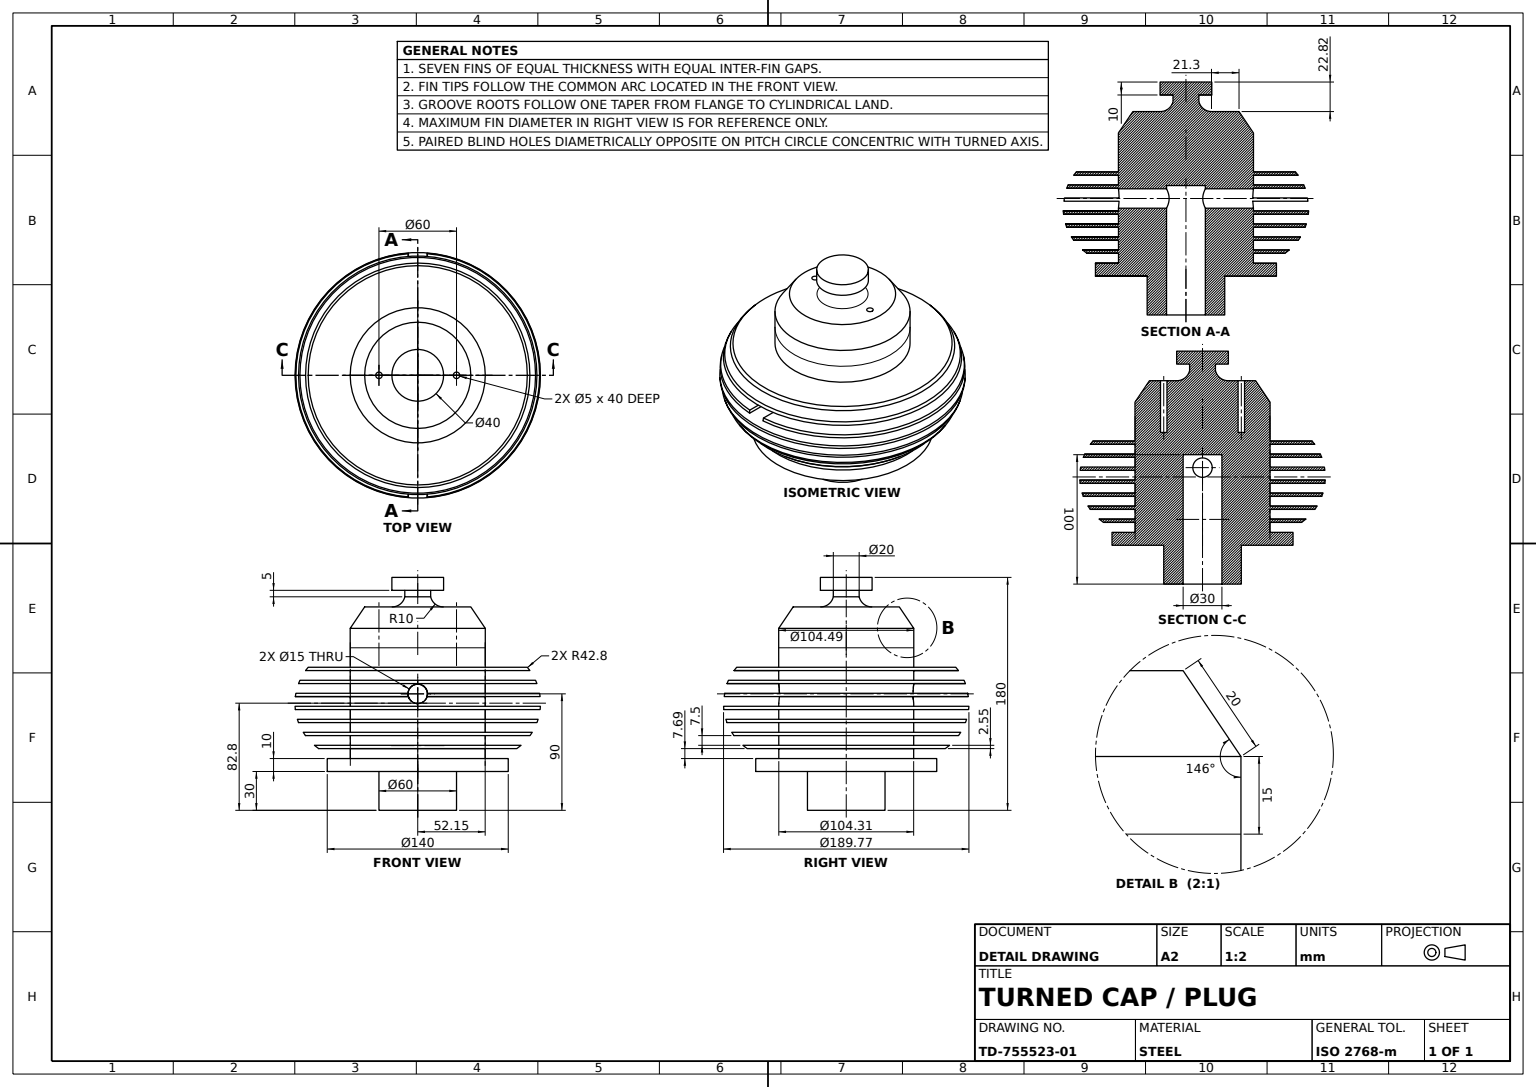
from build123d import *

# Parameters (mm, degrees)
CUT_30_SKETCH_R               = 15
CUT_30_DEPTH                  = 100
RECTANGULAR_CUT_SKETCH_R      = 2.5
RECTANGULAR_CUT_40_DEEP_DEPTH = 40
FRONT_PLANE_CUT_DEPTH         = 204.841147396
FRONT_PLANE_CUT_DEPTH_BACK    = 204.841147396
FRONT_PLANE_CUT_SKETCH_R      = 7.5


with BuildPart() as part:
    # Turned Body Profile → Turned Body (revolve)
    with BuildSketch(Plane.XY, mode=Mode.PRIVATE) as turned_body_sk:
        with BuildLine():
            Line((20, 26.558355194), (0, 26.558355194))
            Line((0, 26.558355194), (0, -153.441644806))
            Line((0, -153.441644806), (30, -153.441644806))
            Line((30, -153.441644806), (30, -123.441644806))
            Line((30, -123.441644806), (70, -123.441644806))
            Line((70, -123.441644806), (70, -113.441644806))
            Line((70, -113.441644806), (52.154011426, -113.441644806))
            Line((52.154011426, -113.441644806), (52.162025925, -105.749506337))
            Line((52.162025925, -105.749506337), (76.634167854, -105.749506337))
            ThreePointArc((76.634167854, -105.749506337), (78.316646551, -104.51429636), (79.93690532, -103.198530512))
            Line((79.93690532, -103.198530512), (52.164683807, -103.198530512))
            Line((52.164683807, -103.198530512), (52.17249811, -95.698535939))
            Line((52.17249811, -95.698535939), (86.852602272, -95.698535939))
            ThreePointArc((86.852602272, -95.698535939), (87.728678054, -94.438348239), (88.559008008, -93.147560114))
            Line((88.559008008, -93.147560114), (52.175155992, -93.147560114))
            Line((52.175155992, -93.147560114), (52.182970295, -85.647565542))
            Line((52.182970295, -85.647565542), (92.237204199, -85.647565542))
            ThreePointArc((92.237204199, -85.647565542), (92.689531284, -84.378879966), (93.101714014, -83.096589717))
            Line((93.101714014, -83.096589717), (52.185628177, -83.096589717))
            Line((52.185628177, -83.096589717), (52.19344248, -75.596595145))
            Line((52.19344248, -75.596595145), (94.666226931, -75.596595145))
            ThreePointArc((94.666226931, -75.596595145), (94.795416565, -74.322754392), (94.88644532, -73.04561932))
            Line((94.88644532, -73.04561932), (52.196100362, -73.04561932))
            Line((52.196100362, -73.04561932), (52.203914665, -65.545624748))
            Line((52.203914665, -65.545624748), (94.649547422, -65.545624748))
            ThreePointArc((94.649547422, -65.545624748), (94.476664711, -64.267241391), (94.265333585, -62.994648923))
            Line((94.265333585, -62.994648923), (52.206572547, -62.994648923))
            Line((52.206572547, -62.994648923), (52.21438685, -55.49465435))
            Line((52.21438685, -55.49465435), (92.184108605, -55.49465435))
            ThreePointArc((92.184108605, -55.49465435), (91.674398419, -54.210606739), (91.123512187, -52.943678525))
            Line((91.123512187, -52.943678525), (52.217044732, -52.943678525))
            Line((52.217044732, -52.943678525), (52.224859035, -45.443683953))
            Line((52.224859035, -45.443683953), (86.750294013, -45.443683953))
            ThreePointArc((86.750294013, -45.443683953), (85.769276316, -44.149118192), (84.73984444, -42.892708128))
            Line((84.73984444, -42.892708128), (52.227516917, -42.892708128))
            Line((52.227516917, -42.892708128), (52.23533122, -35.392713556))
            Line((52.23533122, -35.392713556), (52.237989102, -32.841737731))
            Line((52.237989102, -32.841737731), (52.243198641, -27.841737731))
            Line((52.243198641, -27.841737731), (52.243198641, -12.841737731))
            Line((52.243198641, -12.841737731), (41.059340572, 3.73901372))
            Line((41.059340572, 3.73901372), (19.759340572, 3.73901372))
            ThreePointArc((19.759340572, 3.73901372), (13.506604581, 5.934957555), (10, 11.558355194))
            Line((10, 11.558355194), (10, 16.558355194))
            Line((10, 16.558355194), (20, 16.558355194))
            Line((20, 16.558355194), (20, 26.558355194))
        make_face()
    revolve(turned_body_sk.sketch.rotate(Axis((0, 35.480114724, 0), (0, -1, 0)), 180), axis=Axis((0, 35.480114724, 0), (0, -1, 0)))

    # Cut Ø30 Sketch → Cut Ø30 (cut)
    with BuildSketch(Plane.XZ.offset(153.441644806)):
        Circle(CUT_30_SKETCH_R)
    extrude(amount=-CUT_30_DEPTH, mode=Mode.SUBTRACT)

    # Rectangular Cut Sketch → Rectangular Cut 40 Deep (cut)
    with BuildSketch(Plane(origin=(0, 3.73901372, 0), x_dir=(1, 0, 0), z_dir=(0, 1, 0))):
        with Locations(Location((30, 0, 0), (0, 0, 180))):
            Circle(RECTANGULAR_CUT_SKETCH_R)
        with Locations(Location((-30, 0, 0), (0, 0, 180))):
            Circle(RECTANGULAR_CUT_SKETCH_R)
    extrude(amount=-RECTANGULAR_CUT_40_DEEP_DEPTH, mode=Mode.SUBTRACT)

    # Front Plane Cut Sketch → Front Plane Cut (cut, two sides: drawn at the far end of the back side and taken through both)
    with BuildSketch(Plane.XY.offset(-FRONT_PLANE_CUT_DEPTH_BACK)):
        with Locations((0, -63.441644806)):
            Circle(FRONT_PLANE_CUT_SKETCH_R)
    extrude(amount=FRONT_PLANE_CUT_DEPTH + FRONT_PLANE_CUT_DEPTH_BACK, mode=Mode.SUBTRACT)


solid = part.part
